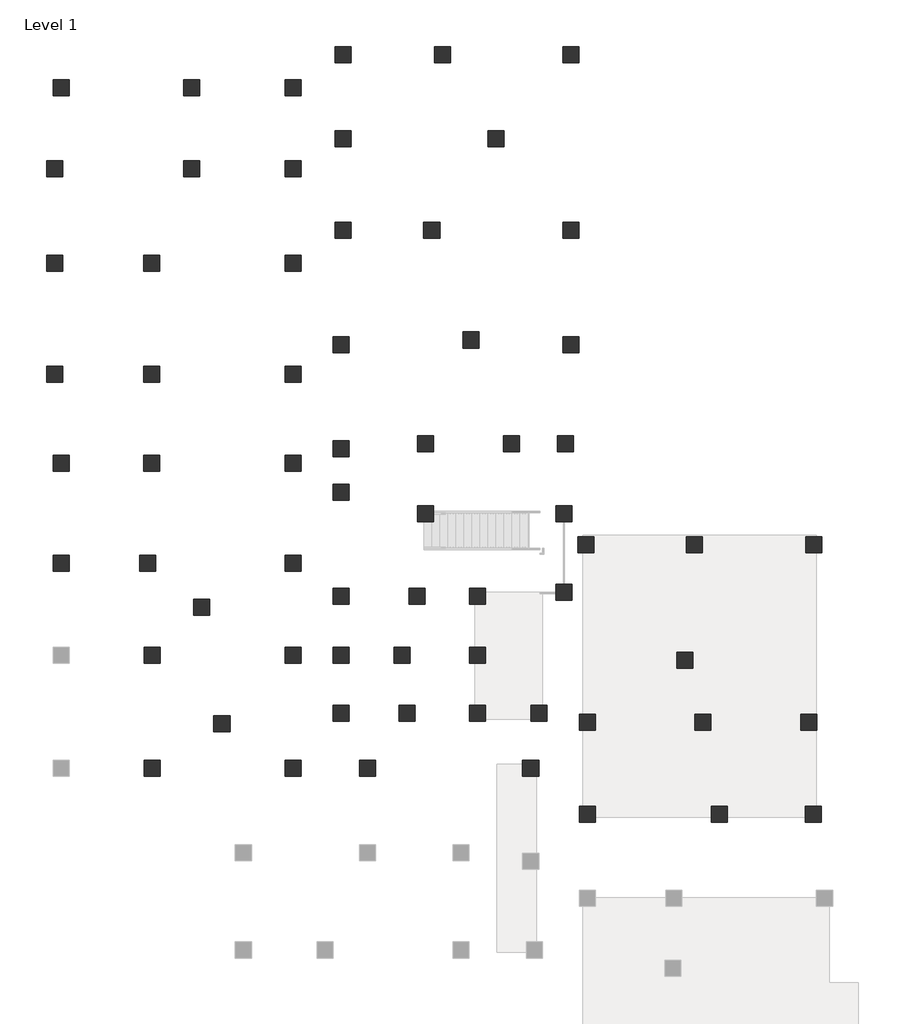
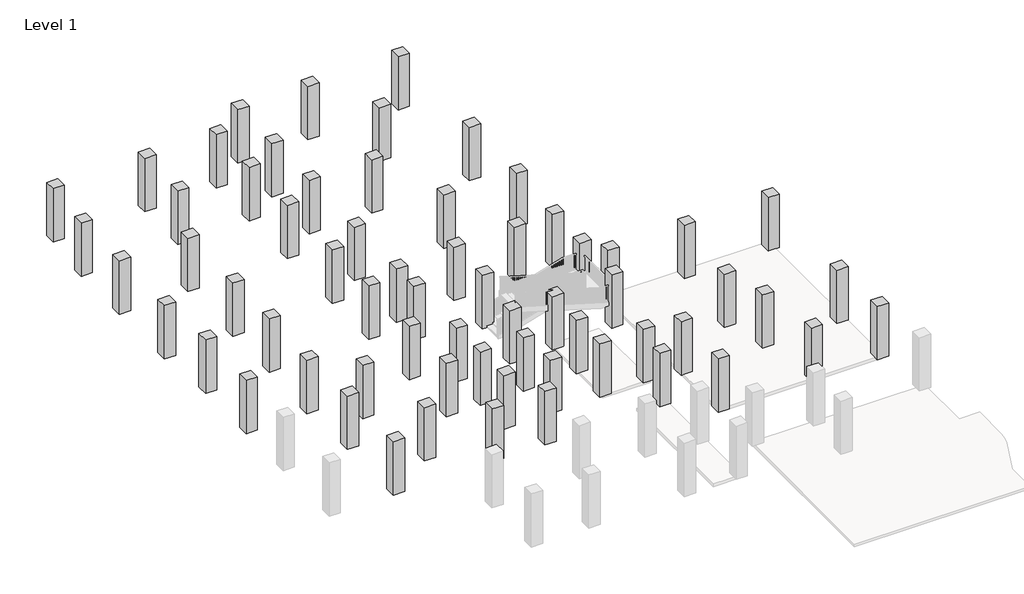
# One storey, part 2 of 6: 65 columns.
"""IFC4 building model written with IfcOpenShell, lengths in millimetres."""

from ifc_helpers import new_model, si_unit, origin, origin_with_axes, place, context, project, spatial, polyline, outline, extrude, element, save

model = new_model("IFC4")

# Units and contexts
model_context = context("Model", 3, world=origin())
ifc_project = project(units=[si_unit("LENGTHUNIT", "METRE", prefix="MILLI")], contexts=[model_context])

# Site, building, storey
site = spatial("IfcSite", under=ifc_project)
building = spatial("IfcBuilding", under=site)
storey = spatial("IfcBuildingStorey", under=building, Name="Level 1", Elevation=0.0)

# Columns
placement = place(None, origin())
element("IfcColumn", 1, ObjectType="Rectangular Column : 24\" x 24\"", at=placement, inside=storey, context=model_context, shape_type="SweptSolid", body=[
    extrude(outline(polyline([(1268.975651, 1350.7469419), (1268.975651, 741.1469419), (659.375651, 741.1469419), (659.375651, 1350.7469419), (1268.975651, 1350.7469419)])), origin_with_axes(), (0.0, 0.0, 1.0), 3048.0),
])
element("IfcColumn", 2, ObjectType="Rectangular Column : 24\" x 24\"", at=placement, inside=storey, context=model_context, shape_type="SweptSolid", body=[
    extrude(outline(polyline([(9867.581954, 1350.7469419), (9867.581954, 741.1469419), (9257.981954, 741.1469419), (9257.981954, 1350.7469419), (9867.581954, 1350.7469419)])), origin_with_axes(), (0.0, 0.0, 1.0), 3048.0),
])
element("IfcColumn", 3, ObjectType="Rectangular Column : 24\" x 24\"", at=placement, inside=storey, context=model_context, shape_type="SweptSolid", body=[
    extrude(outline(polyline([(6291.0788826, 1350.7469419), (6291.0788826, 741.1469419), (5681.4788826, 741.1469419), (5681.4788826, 1350.7469419), (6291.0788826, 1350.7469419)])), origin_with_axes(), (0.0, 0.0, 1.0), 3048.0),
])
element("IfcColumn", 4, ObjectType="Rectangular Column : 24\" x 24\"", at=placement, inside=storey, context=model_context, shape_type="SweptSolid", body=[
    extrude(outline(polyline([(-881.5354844, 3108.0299865), (-881.5354844, 2498.4299865), (-1491.1354844, 2498.4299865), (-1491.1354844, 3108.0299865), (-881.5354844, 3108.0299865)])), origin_with_axes(), (0.0, 0.0, 1.0), 3048.0),
])
element("IfcColumn", 5, ObjectType="Rectangular Column : 24\" x 24\"", at=placement, inside=storey, context=model_context, shape_type="SweptSolid", body=[
    extrude(outline(polyline([(-9923.117594, 3108.0299865), (-9923.117594, 2498.4299865), (-10532.717594, 2498.4299865), (-10532.717594, 3108.0299865), (-9923.117594, 3108.0299865)])), origin_with_axes(), (0.0, 0.0, 1.0), 3048.0),
])
element("IfcColumn", 6, ObjectType="Rectangular Column : 24\" x 24\"", at=placement, inside=storey, context=model_context, shape_type="SweptSolid", body=[
    extrude(outline(polyline([(-7086.8650855, 3108.0299865), (-7086.8650855, 2498.4299865), (-7696.4650855, 2498.4299865), (-7696.4650855, 3108.0299865), (-7086.8650855, 3108.0299865)])), origin_with_axes(), (0.0, 0.0, 1.0), 3048.0),
])
element("IfcColumn", 7, ObjectType="Rectangular Column : 24\" x 24\"", at=placement, inside=storey, context=model_context, shape_type="SweptSolid", body=[
    extrude(outline(polyline([(-15274.7301461, 3108.0299865), (-15274.7301461, 2498.4299865), (-15884.3301461, 2498.4299865), (-15884.3301461, 3108.0299865), (-15274.7301461, 3108.0299865)])), origin_with_axes(), (0.0, 0.0, 1.0), 3048.0),
])
element("IfcColumn", 8, ObjectType="Rectangular Column : 24\" x 24\"", at=placement, inside=storey, context=model_context, shape_type="SweptSolid", body=[
    extrude(outline(polyline([(-15274.7301461, 7403.6904836), (-15274.7301461, 6794.0904836), (-15884.3301461, 6794.0904836), (-15884.3301461, 7403.6904836), (-15274.7301461, 7403.6904836)])), origin_with_axes(), (0.0, 0.0, 1.0), 3048.0),
])
element("IfcColumn", 9, ObjectType="Rectangular Column : 24\" x 24\"", at=placement, inside=storey, context=model_context, shape_type="SweptSolid", body=[
    extrude(outline(polyline([(-9923.117594, 7403.6904836), (-9923.117594, 6794.0904836), (-10532.717594, 6794.0904836), (-10532.717594, 7403.6904836), (-9923.117594, 7403.6904836)])), origin_with_axes(), (0.0, 0.0, 1.0), 3048.0),
])
element("IfcColumn", 10, ObjectType="Rectangular Column : 24\" x 24\"", at=placement, inside=storey, context=model_context, shape_type="SweptSolid", body=[
    extrude(outline(polyline([(-12627.4859686, 4788.1498291), (-12627.4859686, 4178.5498291), (-13237.0859686, 4178.5498291), (-13237.0859686, 4788.1498291), (-12627.4859686, 4788.1498291)])), origin_with_axes(), (0.0, 0.0, 1.0), 3048.0),
])
element("IfcColumn", 11, ObjectType="Rectangular Column : 24\" x 24\"", at=placement, inside=storey, context=model_context, shape_type="SweptSolid", body=[
    extrude(outline(polyline([(-9923.117594, 10887.909652), (-9923.117594, 10278.309652), (-10532.717594, 10278.309652), (-10532.717594, 10887.909652), (-9923.117594, 10887.909652)])), origin_with_axes(), (0.0, 0.0, 1.0), 3048.0),
])
element("IfcColumn", 12, ObjectType="Rectangular Column : 24\" x 24\"", at=placement, inside=storey, context=model_context, shape_type="SweptSolid", body=[
    extrude(outline(polyline([(-18736.0019082, 14689.5583639), (-18736.0019082, 14079.9583639), (-19345.6019082, 14079.9583639), (-19345.6019082, 14689.5583639), (-18736.0019082, 14689.5583639)])), origin_with_axes(), (0.0, 0.0, 1.0), 3048.0),
])
element("IfcColumn", 13, ObjectType="Rectangular Column : 24\" x 24\"", at=placement, inside=storey, context=model_context, shape_type="SweptSolid", body=[
    extrude(outline(polyline([(-9923.117594, 14689.5583639), (-9923.117594, 14079.9583639), (-10532.717594, 14079.9583639), (-10532.717594, 14689.5583639), (-9923.117594, 14689.5583639)])), origin_with_axes(), (0.0, 0.0, 1.0), 3048.0),
])
element("IfcColumn", 14, ObjectType="Rectangular Column : 24\" x 24\"", at=placement, inside=storey, context=model_context, shape_type="SweptSolid", body=[
    extrude(outline(polyline([(-18736.0019082, 10887.909652), (-18736.0019082, 10278.309652), (-19345.6019082, 10278.309652), (-19345.6019082, 10887.909652), (-18736.0019082, 10887.909652)])), origin_with_axes(), (0.0, 0.0, 1.0), 3048.0),
])
element("IfcColumn", 15, ObjectType="Rectangular Column : 24\" x 24\"", at=placement, inside=storey, context=model_context, shape_type="SweptSolid", body=[
    extrude(outline(polyline([(-15459.0395683, 10887.909652), (-15459.0395683, 10278.309652), (-16068.6395683, 10278.309652), (-16068.6395683, 10887.909652), (-15459.0395683, 10887.909652)])), origin_with_axes(), (0.0, 0.0, 1.0), 3048.0),
])
element("IfcColumn", 16, ObjectType="Rectangular Column : 24\" x 24\"", at=placement, inside=storey, context=model_context, shape_type="SweptSolid", body=[
    extrude(outline(polyline([(-13400.8805346, 9222.3321744), (-13400.8805346, 8612.7321744), (-14010.4805346, 8612.7321744), (-14010.4805346, 9222.3321744), (-13400.8805346, 9222.3321744)])), origin_with_axes(), (0.0, 0.0, 1.0), 3048.0),
])
element("IfcColumn", 17, ObjectType="Rectangular Column : 24\" x 24\"", at=placement, inside=storey, context=model_context, shape_type="SweptSolid", body=[
    extrude(outline(polyline([(-8103.7807538, 9640.1313069), (-8103.7807538, 9030.5313069), (-8713.3807538, 9030.5313069), (-8713.3807538, 9640.1313069), (-8103.7807538, 9640.1313069)])), origin_with_axes(), (0.0, 0.0, 1.0), 3048.0),
])
element("IfcColumn", 18, ObjectType="Rectangular Column : 24\" x 24\"", at=placement, inside=storey, context=model_context, shape_type="SweptSolid", body=[
    extrude(outline(polyline([(-5202.9083916, 9640.1313069), (-5202.9083916, 9030.5313069), (-5812.5083916, 9030.5313069), (-5812.5083916, 9640.1313069), (-5202.9083916, 9640.1313069)])), origin_with_axes(), (0.0, 0.0, 1.0), 3048.0),
])
element("IfcColumn", 19, ObjectType="Rectangular Column : 24\" x 24\"", at=placement, inside=storey, context=model_context, shape_type="SweptSolid", body=[
    extrude(outline(polyline([(384.7195627, 9792.0084876), (384.7195627, 9182.4084876), (-224.8804373, 9182.4084876), (-224.8804373, 9792.0084876), (384.7195627, 9792.0084876)])), origin_with_axes(), (0.0, 0.0, 1.0), 3048.0),
])
element("IfcColumn", 20, ObjectType="Rectangular Column : 24\" x 24\"", at=placement, inside=storey, context=model_context, shape_type="SweptSolid", body=[
    extrude(outline(polyline([(-564.8878537, 5186.8170526), (-564.8878537, 4577.2170526), (-1174.4878537, 4577.2170526), (-1174.4878537, 5186.8170526), (-564.8878537, 5186.8170526)])), origin_with_axes(), (0.0, 0.0, 1.0), 3048.0),
])
element("IfcColumn", 21, ObjectType="Rectangular Column : 24\" x 24\"", at=placement, inside=storey, context=model_context, shape_type="SweptSolid", body=[
    extrude(outline(polyline([(-2906.2326628, 7403.6904836), (-2906.2326628, 6794.0904836), (-3515.8326628, 6794.0904836), (-3515.8326628, 7403.6904836), (-2906.2326628, 7403.6904836)])), origin_with_axes(), (0.0, 0.0, 1.0), 3048.0),
])
element("IfcColumn", 22, ObjectType="Rectangular Column : 24\" x 24\"", at=placement, inside=storey, context=model_context, shape_type="SweptSolid", body=[
    extrude(outline(polyline([(-5778.2944484, 7403.6904836), (-5778.2944484, 6794.0904836), (-6387.8944484, 6794.0904836), (-6387.8944484, 7403.6904836), (-5778.2944484, 7403.6904836)])), origin_with_axes(), (0.0, 0.0, 1.0), 3048.0),
])
element("IfcColumn", 23, ObjectType="Rectangular Column : 24\" x 24\"", at=placement, inside=storey, context=model_context, shape_type="SweptSolid", body=[
    extrude(outline(polyline([(-8103.7807538, 7403.6904836), (-8103.7807538, 6794.0904836), (-8713.3807538, 6794.0904836), (-8713.3807538, 7403.6904836), (-8103.7807538, 7403.6904836)])), origin_with_axes(), (0.0, 0.0, 1.0), 3048.0),
])
element("IfcColumn", 24, ObjectType="Rectangular Column : 24\" x 24\"", at=placement, inside=storey, context=model_context, shape_type="SweptSolid", body=[
    extrude(outline(polyline([(-8103.7807538, 5186.8170526), (-8103.7807538, 4577.2170526), (-8713.3807538, 4577.2170526), (-8713.3807538, 5186.8170526), (-8103.7807538, 5186.8170526)])), origin_with_axes(), (0.0, 0.0, 1.0), 3048.0),
])
element("IfcColumn", 25, ObjectType="Rectangular Column : 24\" x 24\"", at=placement, inside=storey, context=model_context, shape_type="SweptSolid", body=[
    extrude(outline(polyline([(-5589.6188567, 5186.8170526), (-5589.6188567, 4577.2170526), (-6199.2188567, 4577.2170526), (-6199.2188567, 5186.8170526), (-5589.6188567, 5186.8170526)])), origin_with_axes(), (0.0, 0.0, 1.0), 3048.0),
])
element("IfcColumn", 26, ObjectType="Rectangular Column : 24\" x 24\"", at=placement, inside=storey, context=model_context, shape_type="SweptSolid", body=[
    extrude(outline(polyline([(-2906.2326628, 5186.8170526), (-2906.2326628, 4577.2170526), (-3515.8326628, 4577.2170526), (-3515.8326628, 5186.8170526), (-2906.2326628, 5186.8170526)])), origin_with_axes(), (0.0, 0.0, 1.0), 3048.0),
])
element("IfcColumn", 27, ObjectType="Rectangular Column : 24\" x 24\"", at=placement, inside=storey, context=model_context, shape_type="SweptSolid", body=[
    extrude(outline(polyline([(-2906.2326628, 9640.1313069), (-2906.2326628, 9030.5313069), (-3515.8326628, 9030.5313069), (-3515.8326628, 9640.1313069), (-2906.2326628, 9640.1313069)])), origin_with_axes(), (0.0, 0.0, 1.0), 3048.0),
])
element("IfcColumn", 28, ObjectType="Rectangular Column : 24\" x 24\"", at=placement, inside=storey, context=model_context, shape_type="SweptSolid", body=[
    extrude(outline(polyline([(-8103.7807538, 13594.8221301), (-8103.7807538, 12985.2221301), (-8713.3807538, 12985.2221301), (-8713.3807538, 13594.8221301), (-8103.7807538, 13594.8221301)])), origin_with_axes(), (0.0, 0.0, 1.0), 3048.0),
])
element("IfcColumn", 29, ObjectType="Rectangular Column : 24\" x 24\"", at=placement, inside=storey, context=model_context, shape_type="SweptSolid", body=[
    extrude(outline(polyline([(-8103.7807538, 15253.1939914), (-8103.7807538, 14643.5939914), (-8713.3807538, 14643.5939914), (-8713.3807538, 15253.1939914), (-8103.7807538, 15253.1939914)])), origin_with_axes(), (0.0, 0.0, 1.0), 3048.0),
])
element("IfcColumn", 30, ObjectType="Rectangular Column : 24\" x 24\"", at=placement, inside=storey, context=model_context, shape_type="SweptSolid", body=[
    extrude(outline(polyline([(446.1237924, 15435.4892491), (446.1237924, 14825.8892491), (-163.4762076, 14825.8892491), (-163.4762076, 15435.4892491), (446.1237924, 15435.4892491)])), origin_with_axes(), (0.0, 0.0, 1.0), 3048.0),
])
element("IfcColumn", 31, ObjectType="Rectangular Column : 24\" x 24\"", at=placement, inside=storey, context=model_context, shape_type="SweptSolid", body=[
    extrude(outline(polyline([(-4880.2713731, 12772.4906593), (-4880.2713731, 12162.8906593), (-5489.8713731, 12162.8906593), (-5489.8713731, 12772.4906593), (-4880.2713731, 12772.4906593)])), origin_with_axes(), (0.0, 0.0, 1.0), 3048.0),
])
element("IfcColumn", 32, ObjectType="Rectangular Column : 24\" x 24\"", at=placement, inside=storey, context=model_context, shape_type="SweptSolid", body=[
    extrude(outline(polyline([(384.7195627, 12772.4906593), (384.7195627, 12162.8906593), (-224.8804373, 12162.8906593), (-224.8804373, 12772.4906593), (384.7195627, 12772.4906593)])), origin_with_axes(), (0.0, 0.0, 1.0), 3048.0),
])
element("IfcColumn", 33, ObjectType="Rectangular Column : 24\" x 24\"", at=placement, inside=storey, context=model_context, shape_type="SweptSolid", body=[
    extrude(outline(polyline([(-15296.7462187, 14689.5583639), (-15296.7462187, 14079.9583639), (-15906.3462187, 14079.9583639), (-15906.3462187, 14689.5583639), (-15296.7462187, 14689.5583639)])), origin_with_axes(), (0.0, 0.0, 1.0), 3048.0),
])
element("IfcColumn", 34, ObjectType="Rectangular Column : 24\" x 24\"", at=placement, inside=storey, context=model_context, shape_type="SweptSolid", body=[
    extrude(outline(polyline([(-9923.117594, 18085.7038949), (-9923.117594, 17476.1038949), (-10532.717594, 17476.1038949), (-10532.717594, 18085.7038949), (-9923.117594, 18085.7038949)])), origin_with_axes(), (0.0, 0.0, 1.0), 3048.0),
])
element("IfcColumn", 35, ObjectType="Rectangular Column : 24\" x 24\"", at=placement, inside=storey, context=model_context, shape_type="SweptSolid", body=[
    extrude(outline(polyline([(-15296.7462187, 18085.7038949), (-15296.7462187, 17476.1038949), (-15906.3462187, 17476.1038949), (-15906.3462187, 18085.7038949), (-15296.7462187, 18085.7038949)])), origin_with_axes(), (0.0, 0.0, 1.0), 3048.0),
])
element("IfcColumn", 36, ObjectType="Rectangular Column : 24\" x 24\"", at=placement, inside=storey, context=model_context, shape_type="SweptSolid", body=[
    extrude(outline(polyline([(-18992.8798594, 18085.7038949), (-18992.8798594, 17476.1038949), (-19602.4798594, 17476.1038949), (-19602.4798594, 18085.7038949), (-18992.8798594, 18085.7038949)])), origin_with_axes(), (0.0, 0.0, 1.0), 3048.0),
])
element("IfcColumn", 37, ObjectType="Rectangular Column : 24\" x 24\"", at=placement, inside=storey, context=model_context, shape_type="SweptSolid", body=[
    extrude(outline(polyline([(-18992.8798594, 22305.0700038), (-18992.8798594, 21695.4700038), (-19602.4798594, 21695.4700038), (-19602.4798594, 22305.0700038), (-18992.8798594, 22305.0700038)])), origin_with_axes(), (0.0, 0.0, 1.0), 3048.0),
])
element("IfcColumn", 38, ObjectType="Rectangular Column : 24\" x 24\"", at=placement, inside=storey, context=model_context, shape_type="SweptSolid", body=[
    extrude(outline(polyline([(-9923.117594, 22305.0700038), (-9923.117594, 21695.4700038), (-10532.717594, 21695.4700038), (-10532.717594, 22305.0700038), (-9923.117594, 22305.0700038)])), origin_with_axes(), (0.0, 0.0, 1.0), 3048.0),
])
element("IfcColumn", 39, ObjectType="Rectangular Column : 24\" x 24\"", at=placement, inside=storey, context=model_context, shape_type="SweptSolid", body=[
    extrude(outline(polyline([(-15296.7462187, 22305.0700038), (-15296.7462187, 21695.4700038), (-15906.3462187, 21695.4700038), (-15906.3462187, 22305.0700038), (-15296.7462187, 22305.0700038)])), origin_with_axes(), (0.0, 0.0, 1.0), 3048.0),
])
element("IfcColumn", 40, ObjectType="Rectangular Column : 24\" x 24\"", at=placement, inside=storey, context=model_context, shape_type="SweptSolid", body=[
    extrude(outline(polyline([(-13780.6118174, 25881.5730752), (-13780.6118174, 25271.9730752), (-14390.2118174, 25271.9730752), (-14390.2118174, 25881.5730752), (-13780.6118174, 25881.5730752)])), origin_with_axes(), (0.0, 0.0, 1.0), 3048.0),
])
element("IfcColumn", 41, ObjectType="Rectangular Column : 24\" x 24\"", at=placement, inside=storey, context=model_context, shape_type="SweptSolid", body=[
    extrude(outline(polyline([(-9923.117594, 25881.5730752), (-9923.117594, 25271.9730752), (-10532.717594, 25271.9730752), (-10532.717594, 25881.5730752), (-9923.117594, 25881.5730752)])), origin_with_axes(), (0.0, 0.0, 1.0), 3048.0),
])
element("IfcColumn", 42, ObjectType="Rectangular Column : 24\" x 24\"", at=placement, inside=storey, context=model_context, shape_type="SweptSolid", body=[
    extrude(outline(polyline([(-18992.8798594, 25881.5730752), (-18992.8798594, 25271.9730752), (-19602.4798594, 25271.9730752), (-19602.4798594, 25881.5730752), (-18992.8798594, 25881.5730752)])), origin_with_axes(), (0.0, 0.0, 1.0), 3048.0),
])
element("IfcColumn", 43, ObjectType="Rectangular Column : 24\" x 24\"", at=placement, inside=storey, context=model_context, shape_type="SweptSolid", body=[
    extrude(outline(polyline([(-18735.3832505, 28959.7902891), (-18735.3832505, 28350.1902891), (-19344.9832505, 28350.1902891), (-19344.9832505, 28959.7902891), (-18735.3832505, 28959.7902891)])), origin_with_axes(), (0.0, 0.0, 1.0), 3048.0),
])
element("IfcColumn", 44, ObjectType="Rectangular Column : 24\" x 24\"", at=placement, inside=storey, context=model_context, shape_type="SweptSolid", body=[
    extrude(outline(polyline([(-13780.6118174, 28959.7902891), (-13780.6118174, 28350.1902891), (-14390.2118174, 28350.1902891), (-14390.2118174, 28959.7902891), (-13780.6118174, 28959.7902891)])), origin_with_axes(), (0.0, 0.0, 1.0), 3048.0),
])
element("IfcColumn", 45, ObjectType="Rectangular Column : 24\" x 24\"", at=placement, inside=storey, context=model_context, shape_type="SweptSolid", body=[
    extrude(outline(polyline([(-9923.117594, 28959.7902891), (-9923.117594, 28350.1902891), (-10532.717594, 28350.1902891), (-10532.717594, 28959.7902891), (-9923.117594, 28959.7902891)])), origin_with_axes(), (0.0, 0.0, 1.0), 3048.0),
])
element("IfcColumn", 46, ObjectType="Rectangular Column : 24\" x 24\"", at=placement, inside=storey, context=model_context, shape_type="SweptSolid", body=[
    extrude(outline(polyline([(-8019.8094041, 30229.6859566), (-8019.8094041, 29620.0859566), (-8629.4094041, 29620.0859566), (-8629.4094041, 30229.6859566), (-8019.8094041, 30229.6859566)])), origin_with_axes(), (0.0, 0.0, 1.0), 3048.0),
])
element("IfcColumn", 47, ObjectType="Rectangular Column : 24\" x 24\"", at=placement, inside=storey, context=model_context, shape_type="SweptSolid", body=[
    extrude(outline(polyline([(-4229.1707744, 30229.6859566), (-4229.1707744, 29620.0859566), (-4838.7707744, 29620.0859566), (-4838.7707744, 30229.6859566), (-4229.1707744, 30229.6859566)])), origin_with_axes(), (0.0, 0.0, 1.0), 3048.0),
])
element("IfcColumn", 48, ObjectType="Rectangular Column : 24\" x 24\"", at=placement, inside=storey, context=model_context, shape_type="SweptSolid", body=[
    extrude(outline(polyline([(-8019.8094041, 27031.0003474), (-8019.8094041, 26421.4003474), (-8629.4094041, 26421.4003474), (-8629.4094041, 27031.0003474), (-8019.8094041, 27031.0003474)])), origin_with_axes(), (0.0, 0.0, 1.0), 3048.0),
])
element("IfcColumn", 49, ObjectType="Rectangular Column : 24\" x 24\"", at=placement, inside=storey, context=model_context, shape_type="SweptSolid", body=[
    extrude(outline(polyline([(-8019.8094041, 23550.9838773), (-8019.8094041, 22941.3838773), (-8629.4094041, 22941.3838773), (-8629.4094041, 23550.9838773), (-8019.8094041, 23550.9838773)])), origin_with_axes(), (0.0, 0.0, 1.0), 3048.0),
])
element("IfcColumn", 50, ObjectType="Rectangular Column : 24\" x 24\"", at=placement, inside=storey, context=model_context, shape_type="SweptSolid", body=[
    extrude(outline(polyline([(-8103.7807538, 19190.4813122), (-8103.7807538, 18580.8813122), (-8713.3807538, 18580.8813122), (-8713.3807538, 19190.4813122), (-8103.7807538, 19190.4813122)])), origin_with_axes(), (0.0, 0.0, 1.0), 3048.0),
])
element("IfcColumn", 51, ObjectType="Rectangular Column : 24\" x 24\"", at=placement, inside=storey, context=model_context, shape_type="SweptSolid", body=[
    extrude(outline(polyline([(-3149.3522242, 19379.156904), (-3149.3522242, 18769.556904), (-3758.9522242, 18769.556904), (-3758.9522242, 19379.156904), (-3149.3522242, 19379.156904)])), origin_with_axes(), (0.0, 0.0, 1.0), 3048.0),
])
element("IfcColumn", 52, ObjectType="Rectangular Column : 24\" x 24\"", at=placement, inside=storey, context=model_context, shape_type="SweptSolid", body=[
    extrude(outline(polyline([(645.1235656, 19190.4813122), (645.1235656, 18580.8813122), (35.5235656, 18580.8813122), (35.5235656, 19190.4813122), (645.1235656, 19190.4813122)])), origin_with_axes(), (0.0, 0.0, 1.0), 3048.0),
])
element("IfcColumn", 53, ObjectType="Rectangular Column : 24\" x 24\"", at=placement, inside=storey, context=model_context, shape_type="SweptSolid", body=[
    extrude(outline(polyline([(645.1235656, 23550.9838773), (645.1235656, 22941.3838773), (35.5235656, 22941.3838773), (35.5235656, 23550.9838773), (645.1235656, 23550.9838773)])), origin_with_axes(), (0.0, 0.0, 1.0), 3048.0),
])
element("IfcColumn", 54, ObjectType="Rectangular Column : 24\" x 24\"", at=placement, inside=storey, context=model_context, shape_type="SweptSolid", body=[
    extrude(outline(polyline([(-4645.1303877, 23550.9838773), (-4645.1303877, 22941.3838773), (-5254.7303877, 22941.3838773), (-5254.7303877, 23550.9838773), (-4645.1303877, 23550.9838773)])), origin_with_axes(), (0.0, 0.0, 1.0), 3048.0),
])
element("IfcColumn", 55, ObjectType="Rectangular Column : 24\" x 24\"", at=placement, inside=storey, context=model_context, shape_type="SweptSolid", body=[
    extrude(outline(polyline([(645.1235656, 30229.6859566), (645.1235656, 29620.0859566), (35.5235656, 29620.0859566), (35.5235656, 30229.6859566), (645.1235656, 30229.6859566)])), origin_with_axes(), (0.0, 0.0, 1.0), 3048.0),
])
element("IfcColumn", 56, ObjectType="Rectangular Column : 24\" x 24\"", at=placement, inside=storey, context=model_context, shape_type="SweptSolid", body=[
    extrude(outline(polyline([(-2210.1670563, 27031.0003474), (-2210.1670563, 26421.4003474), (-2819.7670563, 26421.4003474), (-2819.7670563, 27031.0003474), (-2210.1670563, 27031.0003474)])), origin_with_axes(), (0.0, 0.0, 1.0), 3048.0),
])
element("IfcColumn", 57, ObjectType="Rectangular Column : 24\" x 24\"", at=placement, inside=storey, context=model_context, shape_type="SweptSolid", body=[
    extrude(outline(polyline([(1225.3714407, 11595.7088895), (1225.3714407, 10986.1088895), (615.7714407, 10986.1088895), (615.7714407, 11595.7088895), (1225.3714407, 11595.7088895)])), origin_with_axes(), (0.0, 0.0, 1.0), 3048.0),
])
element("IfcColumn", 58, ObjectType="Rectangular Column : 24\" x 24\"", at=placement, inside=storey, context=model_context, shape_type="SweptSolid", body=[
    extrude(outline(polyline([(9884.3961832, 11595.7088895), (9884.3961832, 10986.1088895), (9274.7961832, 10986.1088895), (9274.7961832, 11595.7088895), (9884.3961832, 11595.7088895)])), origin_with_axes(), (0.0, 0.0, 1.0), 3048.0),
])
element("IfcColumn", 59, ObjectType="Rectangular Column : 24\" x 24\"", at=placement, inside=storey, context=model_context, shape_type="SweptSolid", body=[
    extrude(outline(polyline([(5345.2442656, 11595.7088895), (5345.2442656, 10986.1088895), (4735.6442656, 10986.1088895), (4735.6442656, 11595.7088895), (5345.2442656, 11595.7088895)])), origin_with_axes(), (0.0, 0.0, 1.0), 3048.0),
])
element("IfcColumn", 60, ObjectType="Rectangular Column : 24\" x 24\"", at=placement, inside=storey, context=model_context, shape_type="SweptSolid", body=[
    extrude(outline(polyline([(4980.6537501, 7202.3931781), (4980.6537501, 6592.7931781), (4371.0537501, 6592.7931781), (4371.0537501, 7202.3931781), (4980.6537501, 7202.3931781)])), origin_with_axes(), (0.0, 0.0, 1.0), 3048.0),
])
element("IfcColumn", 61, ObjectType="Rectangular Column : 24\" x 24\"", at=placement, inside=storey, context=model_context, shape_type="SweptSolid", body=[
    extrude(outline(polyline([(1280.0600181, 4850.7843533), (1280.0600181, 4241.1843533), (670.4600181, 4241.1843533), (670.4600181, 4850.7843533), (1280.0600181, 4850.7843533)])), origin_with_axes(), (0.0, 0.0, 1.0), 3048.0),
])
element("IfcColumn", 62, ObjectType="Rectangular Column : 24\" x 24\"", at=placement, inside=storey, context=model_context, shape_type="SweptSolid", body=[
    extrude(outline(polyline([(5673.3757295, 4850.7843533), (5673.3757295, 4241.1843533), (5063.7757295, 4241.1843533), (5063.7757295, 4850.7843533), (5673.3757295, 4850.7843533)])), origin_with_axes(), (0.0, 0.0, 1.0), 3048.0),
])
element("IfcColumn", 63, ObjectType="Rectangular Column : 24\" x 24\"", at=placement, inside=storey, context=model_context, shape_type="SweptSolid", body=[
    extrude(outline(polyline([(9702.1009254, 4850.7843533), (9702.1009254, 4241.1843533), (9092.5009254, 4241.1843533), (9092.5009254, 4850.7843533), (9702.1009254, 4850.7843533)])), origin_with_axes(), (0.0, 0.0, 1.0), 3048.0),
])
element("IfcColumn", 64, ObjectType="Rectangular Column : 24\" x 24\"", at=placement, inside=storey, context=model_context, shape_type="SweptSolid", body=[
    extrude(outline(polyline([(-4880.2713731, 15435.4892491), (-4880.2713731, 14825.8892491), (-5489.8713731, 14825.8892491), (-5489.8713731, 15435.4892491), (-4880.2713731, 15435.4892491)])), origin_with_axes(), (0.0, 0.0, 1.0), 3048.0),
])
element("IfcColumn", 65, ObjectType="Rectangular Column : 24\" x 24\"", at=placement, inside=storey, context=model_context, shape_type="SweptSolid", body=[
    extrude(outline(polyline([(-1620.0421617, 15435.4892491), (-1620.0421617, 14825.8892491), (-2229.6421617, 14825.8892491), (-2229.6421617, 15435.4892491), (-1620.0421617, 15435.4892491)])), origin_with_axes(), (0.0, 0.0, 1.0), 3048.0),
])

save(model, "model.ifc")

# Revit data of these elements
# Type "Rectangular Column : 24\" x 24\""
#   Assembly Code = "B1010200"
#   Depth = 2' - 0"
#   Offset Base = 0' - 0"
#   Offset Top = 0' - 0"
#   Width = 2' - 0"
#   Material = none
# Elements 1, 3, 6, 10, 16, 20, 32, 38, 47, 48, 51, 53, 54, 56, 57, 59, 61, 62, 65 (IfcColumn, "Rectangular Column : 24\" x 24\"")
#   Phase Created = New Construction
#   Materials on its faces: "Cherry", "Wood - Stained"
# Elements 2, 4, 5, 7, 8, 9, 11, 14, 19, 21, 22, 23, 24, 26, 30, 33, 45, 46, 49, 52, 55, 58, 60, 63, 64 (IfcColumn, "Rectangular Column : 24\" x 24\"")
#   Phase Created = New Construction
#   Materials on its faces: "Wood - Stained", "Cherry"
# Elements 12, 15, 25, 29, 31, 34, 35, 36, 37, 39, 40, 41, 42, 43, 50 (IfcColumn, "Rectangular Column : 24\" x 24\"")
#   Phase Created = New Construction
#   Materials on its faces: "Wood - Stained"
# Elements 13, 17, 18, 27, 28, 44 (IfcColumn, "Rectangular Column : 24\" x 24\"")
#   Phase Created = New Construction
#   Materials on its faces: "Cherry"
# Materials
#   "Cherry": class "Wood", colour RGB 226 177 128, transparency 0, Description = "Prunus Serotina", Cost = 0
#   "Wood - Stained": class "Wood", colour RGB 224 178 126, transparency 0, Cost = 0
